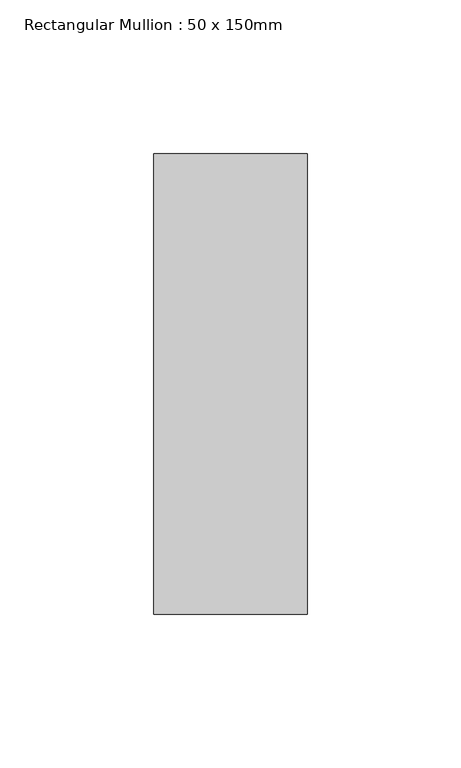
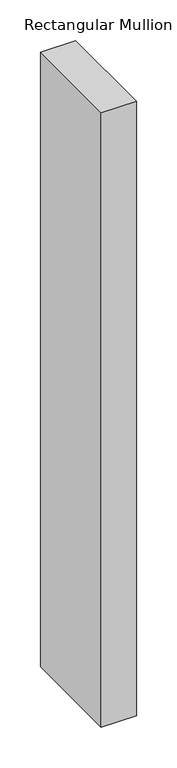
"""IFC4 building model written with IfcOpenShell, lengths in millimetres: member geometry, Rectangular Mullion : 50 x 150mm."""

from ifc_helpers import new_model, si_unit, frame, origin, place, context, project, spatial, polyline, outline, extrude, source, transform, mapped, element, save


def rectangular_mullion_50_x_150mm_a91aaa2b(model_context):
    return source(origin(), model_context, "Body", "SweptSolid", [
        extrude(outline(polyline([(0.0, 75.0), (0.0, -75.0), (-50.0, -75.0), (-50.0, 75.0), (0.0, 75.0)])), frame((0.0, 0.0, -925.0), z_axis=(0.0, 0.0, 1.0), x_axis=(1.0, 0.0, 0.0)), (0.0, 0.0, 1.0), 925.0),
    ])


if __name__ == "__main__":
    model = new_model("IFC4")
    model_context = context("Model", 3, world=origin())
    ifc_project = project(units=[si_unit("LENGTHUNIT", "METRE", prefix="MILLI")], contexts=[model_context])
    site = spatial("IfcSite", under=ifc_project)
    building = spatial("IfcBuilding", under=site)
    placement = place(None, origin())
    rectangular_mullion_50_x_150mm_shape = rectangular_mullion_50_x_150mm_a91aaa2b(model_context)
    element("IfcMember", 1, ObjectType="Rectangular Mullion : 50 x 150mm", at=placement, inside=building, context=model_context, shape_type="MappedRepresentation", body=[
        mapped(rectangular_mullion_50_x_150mm_shape, transform((0.0, 0.0, 0.0), x_axis=(1.0, 0.0, 0.0), y_axis=(0.0, 1.0, 0.0), z_axis=(0.0, 0.0, 1.0))),
    ])
    save(model, "model.ifc")

# Revit data of these elements
# Type "Rectangular Mullion : 50 x 150mm"
#   built-in parameter 1007304 = 0.492126 (stored number, unit not read)
#   built-in parameter 1007301 = 0.082021 (stored number, unit not read)
#   built-in parameter 1007300 = 0.082021 (stored number, unit not read)
# Element 1 (IfcMember, "Rectangular Mullion : 50 x 150mm")
#   Materials on its faces: "Aluminium"
# Materials
#   "Aluminium": class "Metal", colour RGB 247 247 247, transparency 0, Description = "Aluminium 6061", Cost = 0
